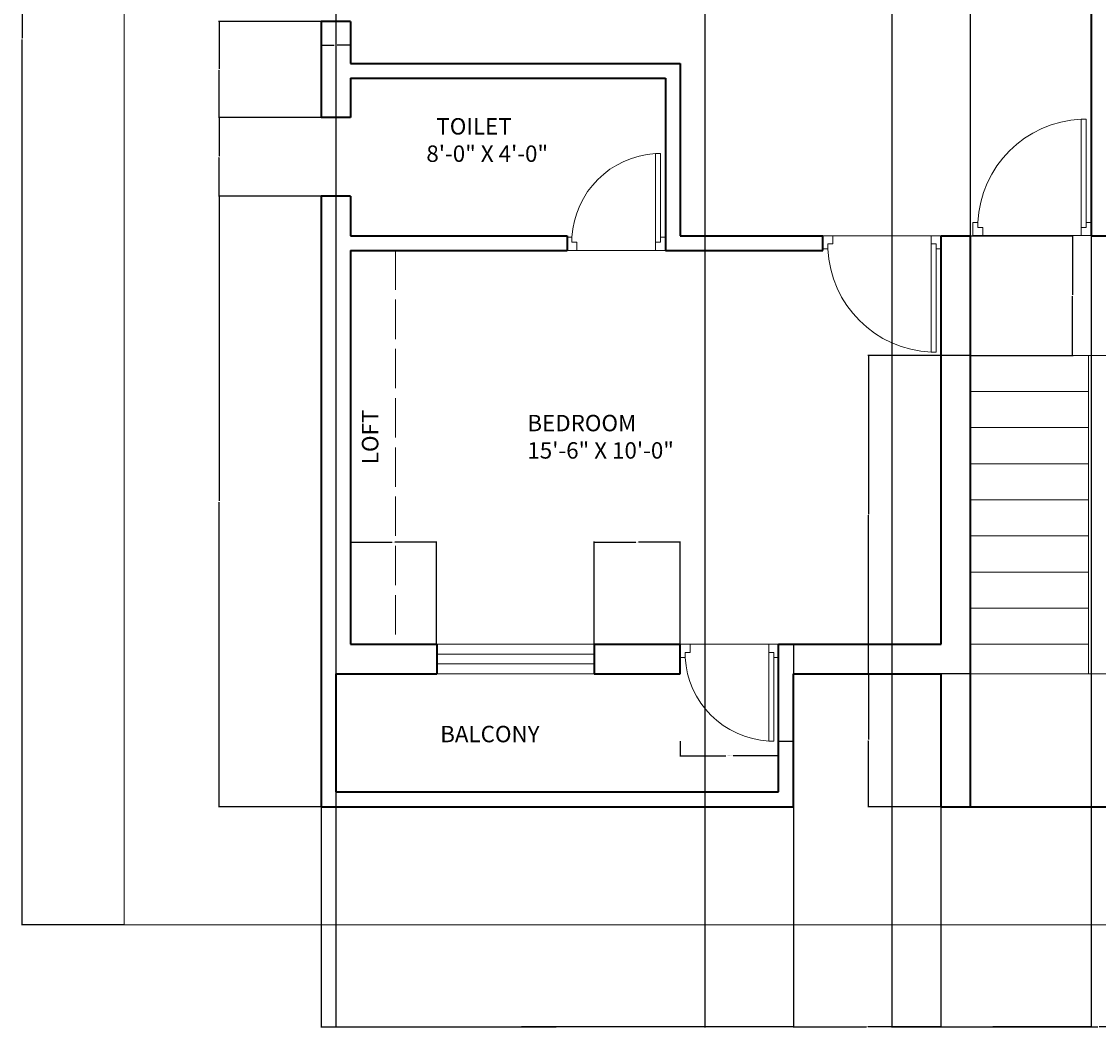
# Model space of a CAD drawing. Units: inches. Extents: x 3263 to 3926, y 954 to 1556.
# Tile 1 of 3: x 3263 to 3592, y 954 to 1260. Entities that reach past the tile are written whole.
import ezdxf

# ---------------------------------------------------------------- set-up
doc = ezdxf.new("R2010")
doc.units = ezdxf.units.IN
doc.linetypes.add('ACAD_ISO02W100', pattern=[15, 12, -3])
for name, color, linetype, lineweight in [('A-ANNO-DIMS', 2, 'Continuous', 18), ('A-ANNO-TEXT', 7, 'Continuous', 18), ('A-AREA-IDEN', 7, 'Continuous', 18), ('A-FLOR-OVHD', 8, 'ACAD_ISO02W100', 13), ('C-PROP', 8, 'Continuous', 18), ('door', 30, 'Continuous', 18), ('staircase', 31, 'Continuous', 18), ('wall', 7, 'Continuous', 35), ('window', 92, 'Continuous', 18)]:
    doc.layers.add(name, color=color, linetype=linetype, lineweight=lineweight)
doc.styles.get("Standard").update_dxf_attribs({"font": 'arial.ttf'})
doc.dimstyles.get("Standard").update_dxf_attribs({"dimtxt": 0.18, "dimasz": 0.18, "dimexe": 0.18, "dimexo": 0.0625, "dimgap": 0.09, "dimtad": 0, "dimtih": 1, "dimtoh": 1, "dimdec": 4, "dimzin": 0, "dimdsep": 46, "dimtxsty": 'Standard', "dimcen": 0.09, "dimadec": 0, "dimazin": 0, "dimtfac": 1, "dimtdec": 4, "dimtofl": 0, "dimtmove": 0, "dimatfit": 3, "dimfxl": 1, "dimtolj": 1, "dimtzin": 0, "dimarcsym": 0})

# ---------------------------------------------------------------- blocks, each defined once
blk = doc.blocks.new('d2')
at = {"layer": 'door'}
blk.add_line((4131.56, 1215.38), (4161.56, 1215.38), dxfattribs=at)
blk.add_lwpolyline([(4133.06, 1217.88), (4134.56, 1217.88), (4134.56, 1244.88), (4133.06, 1244.88)], close=True, dxfattribs=at)
for points in [[(4134.56, 1215.38), (4131.56, 1215.38), (4131.56, 1219.38), (4133.06, 1219.38), (4133.06, 1217.88), (4134.56, 1217.88), (4134.56, 1215.38)], [(4158.56, 1215.38), (4161.56, 1215.38), (4161.56, 1219.38), (4160.06, 1219.38), (4160.06, 1217.88), (4158.56, 1217.88), (4158.56, 1215.38)]]:
    blk.add_lwpolyline(points, dxfattribs=at)
blk.add_arc((4133.06, 1217.88), 27.04, 3.1798, 86.8202, dxfattribs=at)
blk = doc.blocks.new('w1')
at = {"layer": 'window'}
for p, q in [((3981.35, 1421.04), (3981.35, 1373.04)), ((3984.35, 1421.04), (3984.35, 1373.04))]:
    blk.add_line(p, q, dxfattribs=at)
blk.add_lwpolyline([(3978.35, 1373.04), (3987.35, 1373.04), (3987.35, 1421.04), (3978.35, 1421.04)], close=True, dxfattribs=at)
blk = doc.blocks.new('d1')
at = {"layer": 'door'}
blk.add_line((4131.56, 1272.79), (4167.56, 1272.79), dxfattribs=at)
blk.add_lwpolyline([(4133.06, 1275.29), (4134.56, 1275.29), (4134.56, 1308.29), (4133.06, 1308.29)], close=True, dxfattribs=at)
for points in [[(4134.56, 1272.79), (4131.56, 1272.79), (4131.56, 1276.79), (4133.06, 1276.79), (4133.06, 1275.29), (4134.56, 1275.29), (4134.56, 1272.79)], [(4164.56, 1272.79), (4167.56, 1272.79), (4167.56, 1276.79), (4166.06, 1276.79), (4166.06, 1275.29), (4164.56, 1275.29), (4164.56, 1272.79)]]:
    blk.add_lwpolyline(points, dxfattribs=at)
blk.add_arc((4133.06, 1275.29), 33.03, 2.6026, 87.3974, dxfattribs=at)
blk = doc.blocks.new('*D8')
at = {"layer": 'A-ANNO-DIMS', "color": 0, "lineweight": -2, "transparency": 16777216}
for p, q in [((3464.17, 1040.87), (3464.17, 1036.25)), ((3494.17, 1040.87), (3494.17, 1036.25)), ((3464.35, 1036.43), (3478.04, 1036.43)), ((3493.99, 1036.43), (3480.31, 1036.43))]:
    blk.add_line(p, q, dxfattribs=at)
at = {"layer": 'A-ANNO-DIMS', "color": 0, "transparency": 16777216}
for points in [[(3464.35, 1036.46), (3464.35, 1036.4), (3464.17, 1036.43)], [(3493.99, 1036.46), (3493.99, 1036.4), (3494.17, 1036.43)]]:
    blk.add_solid(points, dxfattribs=at)
at = {"layer": 'Defpoints', "color": 0, "transparency": 16777216}
for p in [(3464.17, 1040.93), (3494.17, 1040.93), (3464.17, 1036.43)]:
    blk.add_point(p, dxfattribs=at)
at = {"layer": 'A-ANNO-DIMS', "color": 0, "transparency": 16777216, "insert": (3479.17, 1036.43), "char_height": 0.18, "attachment_point": 5}
blk.add_mtext('\\A1;DOOR D2 30 TYP.', dxfattribs=at)
blk = doc.blocks.new('*D9')
at = {"layer": 'A-ANNO-DIMS', "color": 0, "lineweight": -2, "transparency": 16777216}
for p, q in [((3494.24, 1070.43), (3498.85, 1070.43)), ((3498.67, 1070.25), (3498.67, 1055.86)), ((3498.67, 1041.11), (3498.67, 1055.5)), ((3494.24, 1040.93), (3498.85, 1040.93))]:
    blk.add_line(p, q, dxfattribs=at)
at = {"layer": 'A-ANNO-DIMS', "color": 0, "transparency": 16777216}
for points in [[(3498.64, 1070.25), (3498.7, 1070.25), (3498.67, 1070.43)], [(3498.64, 1041.11), (3498.7, 1041.11), (3498.67, 1040.93)]]:
    blk.add_solid(points, dxfattribs=at)
at = {"layer": 'Defpoints', "color": 0, "transparency": 16777216}
for p in [(3494.17, 1070.43), (3494.17, 1040.93), (3498.67, 1040.93)]:
    blk.add_point(p, dxfattribs=at)
at = {"layer": 'A-ANNO-DIMS', "color": 0, "transparency": 16777216, "insert": (3498.67, 1055.68), "char_height": 0.18, "attachment_point": 5}
blk.add_mtext('\\A1;30 TYP.', dxfattribs=at)
blk = doc.blocks.new('*D11')
at = {"layer": 'A-ANNO-DIMS', "color": 0, "lineweight": -2, "transparency": 16777216}
for p, q in [((3354.67, 1260.12), (3354.67, 1252.8)), ((3363.67, 1260.12), (3363.67, 1252.8)), ((3354.85, 1252.98), (3358.72, 1252.98)), ((3363.49, 1252.98), (3359.63, 1252.98))]:
    blk.add_line(p, q, dxfattribs=at)
at = {"layer": 'A-ANNO-DIMS', "color": 0, "transparency": 16777216}
for points in [[(3354.85, 1253.01), (3354.85, 1252.95), (3354.67, 1252.98)], [(3363.49, 1253.01), (3363.49, 1252.95), (3363.67, 1252.98)]]:
    blk.add_solid(points, dxfattribs=at)
at = {"layer": 'Defpoints', "color": 0, "transparency": 16777216}
for p in [(3354.67, 1260.18), (3363.67, 1260.18), (3363.67, 1252.98)]:
    blk.add_point(p, dxfattribs=at)
at = {"layer": 'A-ANNO-DIMS', "color": 0, "transparency": 16777216, "insert": (3359.17, 1252.98), "char_height": 0.18, "attachment_point": 5}
blk.add_mtext('\\A1;9 TYP.', dxfattribs=at)
blk = doc.blocks.new('*D17')
at = {"layer": 'A-ANNO-DIMS', "color": 0, "lineweight": -2, "transparency": 16777216}
for p, q in [((3294.61, 1524.93), (3263.39, 1524.93)), ((3263.57, 1524.75), (3263.57, 1255.11)), ((3263.57, 985.11), (3263.57, 1254.75)), ((3294.61, 984.93), (3263.39, 984.93))]:
    blk.add_line(p, q, dxfattribs=at)
at = {"layer": 'A-ANNO-DIMS', "color": 0, "transparency": 16777216}
for points in [[(3263.54, 1524.75), (3263.6, 1524.75), (3263.57, 1524.93)], [(3263.54, 985.11), (3263.6, 985.11), (3263.57, 984.93)]]:
    blk.add_solid(points, dxfattribs=at)
at = {"layer": 'Defpoints', "color": 0, "transparency": 16777216}
for p in [(3263.57, 1524.93), (3294.67, 1524.93), (3294.67, 984.93)]:
    blk.add_point(p, dxfattribs=at)
at = {"layer": 'A-ANNO-DIMS', "color": 0, "transparency": 16777216, "insert": (3263.57, 1254.93), "char_height": 0.18, "attachment_point": 5}
blk.add_mtext('\\A1;540', dxfattribs=at)
blk = doc.blocks.new('*D24')
at = {"layer": 'A-ANNO-DIMS', "color": 0, "lineweight": -2, "transparency": 16777216}
for p, q in [((3354.67, 1020.87), (3354.67, 953.65)), ((3498.67, 1020.87), (3498.67, 953.65)), ((3354.85, 953.83), (3426.39, 953.83)), ((3498.49, 953.83), (3426.95, 953.83))]:
    blk.add_line(p, q, dxfattribs=at)
at = {"layer": 'A-ANNO-DIMS', "color": 0, "transparency": 16777216}
for points in [[(3354.85, 953.86), (3354.85, 953.8), (3354.67, 953.83)], [(3498.49, 953.86), (3498.49, 953.8), (3498.67, 953.83)]]:
    blk.add_solid(points, dxfattribs=at)
at = {"layer": 'Defpoints', "color": 0, "transparency": 16777216}
for p in [(3354.67, 1020.93), (3498.67, 1020.93), (3498.67, 953.83)]:
    blk.add_point(p, dxfattribs=at)
at = {"layer": 'A-ANNO-DIMS', "color": 0, "transparency": 16777216, "insert": (3426.67, 953.83), "char_height": 0.18, "attachment_point": 5}
blk.add_mtext('\\A1;144', dxfattribs=at)
blk = doc.blocks.new('*D25')
at = {"layer": 'A-ANNO-DIMS', "color": 0, "lineweight": -2, "transparency": 16777216}
for p, q in [((3498.67, 1020.87), (3498.67, 953.65)), ((3543.67, 1020.87), (3543.67, 953.65)), ((3498.85, 953.83), (3520.95, 953.83)), ((3543.49, 953.83), (3521.4, 953.83))]:
    blk.add_line(p, q, dxfattribs=at)
at = {"layer": 'A-ANNO-DIMS', "color": 0, "transparency": 16777216}
for points in [[(3498.85, 953.86), (3498.85, 953.8), (3498.67, 953.83)], [(3543.49, 953.86), (3543.49, 953.8), (3543.67, 953.83)]]:
    blk.add_solid(points, dxfattribs=at)
at = {"layer": 'Defpoints', "color": 0, "transparency": 16777216}
for p in [(3498.67, 1020.93), (3543.67, 1020.93), (3543.67, 953.83)]:
    blk.add_point(p, dxfattribs=at)
at = {"layer": 'A-ANNO-DIMS', "color": 0, "transparency": 16777216, "insert": (3521.17, 953.83), "char_height": 0.18, "attachment_point": 5}
blk.add_mtext('\\A1;45', dxfattribs=at)
blk = doc.blocks.new('*D26')
at = {"layer": 'A-ANNO-DIMS', "color": 0, "lineweight": -2, "transparency": 16777216}
for p, q in [((3543.67, 1020.87), (3543.67, 953.65)), ((3639.67, 1020.87), (3639.67, 953.65)), ((3543.85, 953.83), (3591.46, 953.83)), ((3639.49, 953.83), (3591.89, 953.83))]:
    blk.add_line(p, q, dxfattribs=at)
at = {"layer": 'A-ANNO-DIMS', "color": 0, "transparency": 16777216}
for points in [[(3543.85, 953.86), (3543.85, 953.8), (3543.67, 953.83)], [(3639.49, 953.86), (3639.49, 953.8), (3639.67, 953.83)]]:
    blk.add_solid(points, dxfattribs=at)
at = {"layer": 'Defpoints', "color": 0, "transparency": 16777216}
for p in [(3543.67, 1020.93), (3639.67, 1020.93), (3639.67, 953.83)]:
    blk.add_point(p, dxfattribs=at)
at = {"layer": 'A-ANNO-DIMS', "color": 0, "transparency": 16777216, "insert": (3591.67, 953.83), "char_height": 0.18, "attachment_point": 5}
blk.add_mtext('\\A1;96', dxfattribs=at)
blk = doc.blocks.new('*D29')
at = {"layer": 'A-ANNO-DIMS', "color": 0, "lineweight": -2, "transparency": 16777216}
for p, q in [((3552.67, 1020.99), (3552.67, 1556.21)), ((3630.67, 1020.99), (3630.67, 1556.21)), ((3552.85, 1556.03), (3591.46, 1556.03)), ((3630.49, 1556.03), (3591.89, 1556.03))]:
    blk.add_line(p, q, dxfattribs=at)
at = {"layer": 'A-ANNO-DIMS', "color": 0, "transparency": 16777216}
for points in [[(3552.85, 1556.06), (3552.85, 1556), (3552.67, 1556.03)], [(3630.49, 1556.06), (3630.49, 1556), (3630.67, 1556.03)]]:
    blk.add_solid(points, dxfattribs=at)
at = {"layer": 'Defpoints', "color": 0, "transparency": 16777216}
for p in [(3630.67, 1556.03), (3552.67, 1020.93), (3630.67, 1020.93)]:
    blk.add_point(p, dxfattribs=at)
at = {"layer": 'A-ANNO-DIMS', "color": 0, "transparency": 16777216, "insert": (3591.67, 1556.03), "char_height": 0.18, "attachment_point": 5}
blk.add_mtext('\\A1;78', dxfattribs=at)
blk = doc.blocks.new('*D30')
at = {"layer": 'A-ANNO-DIMS', "color": 0, "lineweight": -2, "transparency": 16777216}
for p, q in [((3552.61, 1158.43), (3521.39, 1158.43)), ((3521.57, 1158.25), (3521.57, 1110.11)), ((3521.57, 1061.61), (3521.57, 1109.75)), ((3552.61, 1061.43), (3521.39, 1061.43))]:
    blk.add_line(p, q, dxfattribs=at)
at = {"layer": 'A-ANNO-DIMS', "color": 0, "transparency": 16777216}
for points in [[(3521.54, 1158.25), (3521.6, 1158.25), (3521.57, 1158.43)], [(3521.54, 1061.61), (3521.6, 1061.61), (3521.57, 1061.43)]]:
    blk.add_solid(points, dxfattribs=at)
at = {"layer": 'Defpoints', "color": 0, "transparency": 16777216}
for p in [(3521.57, 1158.43), (3552.67, 1158.43), (3552.67, 1061.43)]:
    blk.add_point(p, dxfattribs=at)
at = {"layer": 'A-ANNO-DIMS', "color": 0, "transparency": 16777216, "insert": (3521.57, 1109.93), "char_height": 0.18, "attachment_point": 5}
blk.add_mtext('\\A1;97', dxfattribs=at)
blk = doc.blocks.new('*D31')
at = {"layer": 'A-ANNO-DIMS', "color": 0, "lineweight": -2, "transparency": 16777216}
for p, q in [((3552.74, 1194.93), (3583.95, 1194.93)), ((3583.77, 1194.75), (3583.77, 1176.86)), ((3583.77, 1158.61), (3583.77, 1176.5)), ((3552.74, 1158.43), (3583.95, 1158.43))]:
    blk.add_line(p, q, dxfattribs=at)
at = {"layer": 'A-ANNO-DIMS', "color": 0, "transparency": 16777216}
for points in [[(3583.74, 1194.75), (3583.8, 1194.75), (3583.77, 1194.93)], [(3583.74, 1158.61), (3583.8, 1158.61), (3583.77, 1158.43)]]:
    blk.add_solid(points, dxfattribs=at)
at = {"layer": 'Defpoints', "color": 0, "transparency": 16777216}
for p in [(3552.67, 1194.93), (3552.67, 1158.43), (3583.77, 1158.43)]:
    blk.add_point(p, dxfattribs=at)
at = {"layer": 'A-ANNO-DIMS', "color": 0, "transparency": 16777216, "insert": (3583.77, 1176.68), "char_height": 0.18, "attachment_point": 5}
blk.add_mtext('\\A1;36.5', dxfattribs=at)
blk = doc.blocks.new('*D32')
at = {"layer": 'A-ANNO-DIMS', "color": 0, "lineweight": -2, "transparency": 16777216}
for p, q in [((3552.61, 1061.43), (3521.39, 1061.43)), ((3521.57, 1061.25), (3521.57, 1041.36)), ((3521.57, 1021.11), (3521.57, 1041)), ((3552.61, 1020.93), (3521.39, 1020.93))]:
    blk.add_line(p, q, dxfattribs=at)
at = {"layer": 'A-ANNO-DIMS', "color": 0, "transparency": 16777216}
for points in [[(3521.54, 1061.25), (3521.6, 1061.25), (3521.57, 1061.43)], [(3521.54, 1021.11), (3521.6, 1021.11), (3521.57, 1020.93)]]:
    blk.add_solid(points, dxfattribs=at)
at = {"layer": 'Defpoints', "color": 0, "transparency": 16777216}
for p in [(3521.57, 1061.43), (3552.67, 1061.43), (3552.67, 1020.93)]:
    blk.add_point(p, dxfattribs=at)
at = {"layer": 'A-ANNO-DIMS', "color": 0, "transparency": 16777216, "insert": (3521.57, 1041.18), "char_height": 0.18, "attachment_point": 5}
blk.add_mtext('\\A1;40.5', dxfattribs=at)
blk = doc.blocks.new('*D36')
at = {"layer": 'A-ANNO-DIMS', "color": 0, "lineweight": -2, "transparency": 16777216}
for p, q in [((3359.17, 1484.37), (3359.17, 953.65)), ((3471.67, 1484.37), (3471.67, 953.65)), ((3359.35, 953.83), (3415.04, 953.83)), ((3471.49, 953.83), (3415.81, 953.83))]:
    blk.add_line(p, q, dxfattribs=at)
at = {"layer": 'A-ANNO-DIMS', "color": 0, "transparency": 16777216}
for points in [[(3359.35, 953.86), (3359.35, 953.8), (3359.17, 953.83)], [(3471.49, 953.86), (3471.49, 953.8), (3471.67, 953.83)]]:
    blk.add_solid(points, dxfattribs=at)
at = {"layer": 'Defpoints', "color": 0, "transparency": 16777216}
for p in [(3359.17, 1484.43), (3471.67, 1484.43), (3471.67, 953.83)]:
    blk.add_point(p, dxfattribs=at)
at = {"layer": 'A-ANNO-DIMS', "color": 0, "transparency": 16777216, "insert": (3415.42, 953.83), "char_height": 0.18, "attachment_point": 5}
blk.add_mtext('\\A1;112.5', dxfattribs=at)
blk = doc.blocks.new('*D38')
at = {"layer": 'A-ANNO-DIMS', "color": 0, "lineweight": -2, "transparency": 16777216}
for p, q in [((3528.67, 1484.37), (3528.67, 953.65)), ((3589.42, 1484.37), (3589.42, 953.65)), ((3528.85, 953.83), (3558.65, 953.83)), ((3589.24, 953.83), (3559.44, 953.83))]:
    blk.add_line(p, q, dxfattribs=at)
at = {"layer": 'A-ANNO-DIMS', "color": 0, "transparency": 16777216}
for points in [[(3528.85, 953.86), (3528.85, 953.8), (3528.67, 953.83)], [(3589.24, 953.86), (3589.24, 953.8), (3589.42, 953.83)]]:
    blk.add_solid(points, dxfattribs=at)
at = {"layer": 'Defpoints', "color": 0, "transparency": 16777216}
for p in [(3528.67, 1484.43), (3589.42, 1484.43), (3589.42, 953.83)]:
    blk.add_point(p, dxfattribs=at)
at = {"layer": 'A-ANNO-DIMS', "color": 0, "transparency": 16777216, "insert": (3559.05, 953.83), "char_height": 0.18, "attachment_point": 5}
blk.add_mtext('\\A1;60.75', dxfattribs=at)
blk = doc.blocks.new('*D49')
at = {"layer": 'A-ANNO-DIMS', "color": 0, "lineweight": -2, "transparency": 16777216}
for p, q in [((3354.61, 1260.18), (3323.39, 1260.18)), ((3323.57, 1260), (3323.57, 1245.74)), ((3323.57, 1231.11), (3323.57, 1245.37)), ((3354.61, 1230.93), (3323.39, 1230.93))]:
    blk.add_line(p, q, dxfattribs=at)
at = {"layer": 'A-ANNO-DIMS', "color": 0, "transparency": 16777216}
for points in [[(3323.54, 1260), (3323.6, 1260), (3323.57, 1260.18)], [(3323.54, 1231.11), (3323.6, 1231.11), (3323.57, 1230.93)]]:
    blk.add_solid(points, dxfattribs=at)
at = {"layer": 'Defpoints', "color": 0, "transparency": 16777216}
for p in [(3323.57, 1260.18), (3354.67, 1260.18), (3354.67, 1230.93)]:
    blk.add_point(p, dxfattribs=at)
at = {"layer": 'A-ANNO-DIMS', "color": 0, "transparency": 16777216, "insert": (3323.57, 1245.56), "char_height": 0.18, "attachment_point": 5}
blk.add_mtext('\\A1;29.25', dxfattribs=at)
blk = doc.blocks.new('*D50')
at = {"layer": 'A-ANNO-DIMS', "color": 0, "lineweight": -2, "transparency": 16777216}
for p, q in [((3354.61, 1230.93), (3323.39, 1230.93)), ((3323.57, 1230.75), (3323.57, 1219.11)), ((3323.57, 1207.11), (3323.57, 1218.75)), ((3354.61, 1206.93), (3323.39, 1206.93))]:
    blk.add_line(p, q, dxfattribs=at)
at = {"layer": 'A-ANNO-DIMS', "color": 0, "transparency": 16777216}
for points in [[(3323.54, 1230.75), (3323.6, 1230.75), (3323.57, 1230.93)], [(3323.54, 1207.11), (3323.6, 1207.11), (3323.57, 1206.93)]]:
    blk.add_solid(points, dxfattribs=at)
at = {"layer": 'Defpoints', "color": 0, "transparency": 16777216}
for p in [(3323.57, 1230.93), (3354.67, 1230.93), (3354.67, 1206.93)]:
    blk.add_point(p, dxfattribs=at)
at = {"layer": 'A-ANNO-DIMS', "color": 0, "transparency": 16777216, "insert": (3323.57, 1218.93), "char_height": 0.18, "attachment_point": 5}
blk.add_mtext('\\A1;24', dxfattribs=at)
blk = doc.blocks.new('*D51')
at = {"layer": 'A-ANNO-DIMS', "color": 0, "lineweight": -2, "transparency": 16777216}
for p, q in [((3354.61, 1206.93), (3323.39, 1206.93)), ((3323.57, 1206.75), (3323.57, 1114.11)), ((3323.57, 1021.11), (3323.57, 1113.75)), ((3354.61, 1020.93), (3323.39, 1020.93))]:
    blk.add_line(p, q, dxfattribs=at)
at = {"layer": 'A-ANNO-DIMS', "color": 0, "transparency": 16777216}
for points in [[(3323.54, 1206.75), (3323.6, 1206.75), (3323.57, 1206.93)], [(3323.54, 1021.11), (3323.6, 1021.11), (3323.57, 1020.93)]]:
    blk.add_solid(points, dxfattribs=at)
at = {"layer": 'Defpoints', "color": 0, "transparency": 16777216}
for p in [(3323.57, 1206.93), (3354.67, 1206.93), (3354.67, 1020.93)]:
    blk.add_point(p, dxfattribs=at)
at = {"layer": 'A-ANNO-DIMS', "color": 0, "transparency": 16777216, "insert": (3323.57, 1113.93), "char_height": 0.18, "attachment_point": 5}
blk.add_mtext('\\A1;186', dxfattribs=at)
blk = doc.blocks.new('*D52')
at = {"layer": 'A-ANNO-DIMS', "color": 0, "lineweight": -2, "transparency": 16777216}
for p, q in [((3363.67, 1070.49), (3363.67, 1101.71)), ((3363.85, 1101.53), (3376.4, 1101.53)), ((3389.74, 1101.53), (3377.2, 1101.53)), ((3389.92, 1070.49), (3389.92, 1101.71))]:
    blk.add_line(p, q, dxfattribs=at)
at = {"layer": 'A-ANNO-DIMS', "color": 0, "transparency": 16777216}
for points in [[(3363.85, 1101.56), (3363.85, 1101.5), (3363.67, 1101.53)], [(3389.74, 1101.56), (3389.74, 1101.5), (3389.92, 1101.53)]]:
    blk.add_solid(points, dxfattribs=at)
at = {"layer": 'Defpoints', "color": 0, "transparency": 16777216}
for p in [(3389.92, 1101.53), (3363.67, 1070.43), (3389.92, 1070.43)]:
    blk.add_point(p, dxfattribs=at)
at = {"layer": 'A-ANNO-DIMS', "color": 0, "transparency": 16777216, "insert": (3376.8, 1101.53), "char_height": 0.18, "attachment_point": 5}
blk.add_mtext('\\A1;26.25', dxfattribs=at)
blk = doc.blocks.new('*D53')
at = {"layer": 'A-ANNO-DIMS', "color": 0, "lineweight": -2, "transparency": 16777216}
for p, q in [((3437.92, 1070.49), (3437.92, 1101.71)), ((3438.1, 1101.53), (3450.65, 1101.53)), ((3463.99, 1101.53), (3451.45, 1101.53)), ((3464.17, 1070.49), (3464.17, 1101.71))]:
    blk.add_line(p, q, dxfattribs=at)
at = {"layer": 'A-ANNO-DIMS', "color": 0, "transparency": 16777216}
for points in [[(3438.1, 1101.56), (3438.1, 1101.5), (3437.92, 1101.53)], [(3463.99, 1101.56), (3463.99, 1101.5), (3464.17, 1101.53)]]:
    blk.add_solid(points, dxfattribs=at)
at = {"layer": 'Defpoints', "color": 0, "transparency": 16777216}
for p in [(3464.17, 1101.53), (3437.92, 1070.43), (3464.17, 1070.43)]:
    blk.add_point(p, dxfattribs=at)
at = {"layer": 'A-ANNO-DIMS', "color": 0, "transparency": 16777216, "insert": (3451.05, 1101.53), "char_height": 0.18, "attachment_point": 5}
blk.add_mtext('\\A1;26.25', dxfattribs=at)

msp = doc.modelspace()

# ---------------------------------------------------------------- linework, layer by layer
at = {"layer": 'A-FLOR-OVHD'}
msp.add_line((3377.4044, 1190.4303), (3377.4044, 1070.4303), dxfattribs=at)
at = {"layer": 'C-PROP'}
for p, q in [((3294.6743, 1524.9303), (3294.6743, 984.9303)), ((3294.6743, 984.9303), (3894.6743, 984.9303))]:
    msp.add_line(p, q, dxfattribs=at)
at = {"layer": 'staircase'}
for p, q in [((3552.6743, 1158.4303), (3630.6743, 1158.4303)), ((3588.6743, 1061.4303), (3588.6743, 1158.4303)), ((3552.6743, 1147.4303), (3588.6743, 1147.4303)), ((3552.6743, 1136.4303), (3588.6743, 1136.4303)), ((3552.6743, 1125.4303), (3588.6743, 1125.4303)), ((3552.6743, 1114.4303), (3588.6743, 1114.4303)), ((3552.6743, 1103.4303), (3588.6743, 1103.4303)), ((3552.6743, 1092.4303), (3588.6743, 1092.4303)), ((3552.6743, 1081.4303), (3588.6743, 1081.4303)), ((3552.6743, 1070.4303), (3588.6743, 1070.4303)), ((3552.6743, 1061.4303), (3630.6743, 1061.4303))]:
    msp.add_line(p, q, dxfattribs=at)
at = {"layer": 'wall'}
for p, q in [((3589.4243, 1362.9303), (3589.4243, 1194.9303)), ((3363.6743, 1260.1803), (3354.6743, 1260.1803)), ((3354.6743, 1260.1803), (3354.6743, 1230.9303)), ((3363.6743, 1260.1803), (3363.6743, 1247.4303)), ((3363.6743, 1247.4303), (3464.1743, 1247.4303)), ((3464.1743, 1247.4303), (3464.1743, 1194.9303)), ((3363.6743, 1242.9303), (3459.6743, 1242.9303)), ((3363.6743, 1242.9303), (3363.6743, 1230.9303)), ((3459.6743, 1242.9303), (3459.6743, 1190.4303)), ((3363.6743, 1230.9303), (3354.6743, 1230.9303)), ((3363.6743, 1206.9303), (3354.6743, 1206.9303)), ((3354.6743, 1206.9303), (3354.6743, 1020.9303)), ((3363.6743, 1206.9303), (3363.6743, 1194.9303)), ((3363.6743, 1194.9303), (3429.6743, 1194.9303)), ((3429.6743, 1194.9303), (3429.6743, 1190.4303)), ((3464.1743, 1194.9303), (3507.6743, 1194.9303)), ((3507.6743, 1190.4303), (3507.6743, 1194.9303)), ((3543.6743, 1194.9303), (3552.6743, 1194.9303)), ((3543.6743, 1070.4303), (3543.6743, 1194.9303)), ((3552.6743, 1020.9303), (3552.6743, 1194.9303)), ((3589.4243, 1194.9303), (3593.9243, 1194.9303)), ((3363.6743, 1190.4303), (3429.6743, 1190.4303)), ((3363.6743, 1190.4303), (3363.6743, 1070.4303)), ((3459.6743, 1190.4303), (3464.1743, 1190.4303)), ((3464.1743, 1190.4303), (3507.6743, 1190.4303)), ((3363.6743, 1070.4303), (3389.9243, 1070.4303)), ((3389.9243, 1070.4303), (3389.9243, 1061.4303)), ((3437.9243, 1070.4303), (3437.9243, 1061.4303)), ((3437.9243, 1070.4303), (3464.1743, 1070.4303)), ((3464.1743, 1061.4303), (3464.1743, 1070.4303)), ((3494.1743, 1025.4303), (3494.1743, 1070.4303)), ((3494.1743, 1070.4303), (3543.6743, 1070.4303)), ((3359.1743, 1061.4303), (3389.9243, 1061.4303)), ((3359.1743, 1061.4303), (3359.1743, 1025.4303)), ((3437.9243, 1061.4303), (3464.1743, 1061.4303)), ((3498.6743, 1020.9303), (3498.6743, 1061.4303)), ((3498.6743, 1061.4303), (3543.6743, 1061.4303)), ((3543.6743, 1020.9303), (3543.6743, 1061.4303)), ((3359.1743, 1025.4303), (3494.1743, 1025.4303)), ((3354.6743, 1020.9303), (3498.6743, 1020.9303)), ((3543.6743, 1020.9303), (3639.6743, 1020.9303))]:
    msp.add_line(p, q, dxfattribs=at)

# ---------------------------------------------------------------- block references
at = {"layer": 'door', "xscale": -1}
for name, p in [('d1', (7720.9828, -77.8568)), ('d2', (7591.2328, -24.9474))]:
    msp.add_blockref(name, p, dxfattribs=at)
at = {"layer": 'door', "rotation": 180}
for name, p in [('d1', (7675.2328, 2467.7175)), ('d2', (7625.7328, 2285.808))]:
    msp.add_blockref(name, p, dxfattribs=at)
at = {"layer": 'window', "rotation": 270}
msp.add_blockref('w1', (2016.8872, 5048.7852), dxfattribs=at)

# ---------------------------------------------------------------- texts
at = {"layer": 'A-ANNO-TEXT', "insert": (3367.141, 1125.2869), "char_height": 5, "attachment_point": 1, "rotation": 90}
msp.add_mtext_dynamic_manual_height_columns('LOFT', width=62.092631, gutter_width=12.5, heights=[0], dxfattribs=at)
at = {"layer": 'A-AREA-IDEN', "char_height": 5, "attachment_point": 1}
for s, width, insert in [('  TOILET\\P8\'-0" X 4\'-0"', 42.17852, (3386.7807, 1230.7511)), ('BEDROOM\\P15\'-6" X 10\'-0"', 65.299351, (3417.5734, 1140.3257)), ('BALCONY', 62.092631, (3390.9994, 1045.5573))]:
    msp.add_mtext_dynamic_manual_height_columns(s, width=width, gutter_width=12.5, heights=[0], dxfattribs=dict(at, insert=insert))

# ---------------------------------------------------------------- dimensions: what is measured, and where the dimension line sits
at = {"layer": 'A-ANNO-DIMS'}
for base, p1, p2, override, picture, middle in [((3630.6743, 1556.0303), (3552.6743, 1020.9303), (3630.6743, 1020.9303), {"dimdec": 0, "dimlfac": 1, "dimrnd": 0, "dimzin": 0, "dimdsep": 46, "dimlunit": 2}, '*D29', (3591.6743, 1556.0303)), ((3471.6743, 953.8303), (3359.1743, 1484.4303), (3471.6743, 1484.4303), {"dimdec": 1, "dimlfac": 1, "dimrnd": 0, "dimzin": 0, "dimdsep": 46, "dimlunit": 2}, '*D36', (3415.4243, 953.8303)), ((3589.4243, 953.8303), (3528.6743, 1484.4303), (3589.4243, 1484.4303), {"dimdec": 2, "dimlfac": 1, "dimrnd": 0, "dimzin": 0, "dimdsep": 46, "dimlunit": 2}, '*D38', (3559.0493, 953.8303)), ((3389.9243, 1101.5303), (3363.6743, 1070.4303), (3389.9243, 1070.4303), {"dimdec": 2, "dimlfac": 1, "dimrnd": 0, "dimzin": 0, "dimdsep": 46, "dimlunit": 2}, '*D52', (3376.7993, 1101.5303)), ((3498.6743, 953.8303), (3354.6743, 1020.9303), (3498.6743, 1020.9303), {"dimdec": 0, "dimlfac": 1, "dimrnd": 0, "dimzin": 0, "dimdsep": 46, "dimlunit": 2}, '*D24', (3426.6743, 953.8303)), ((3543.6743, 953.8303), (3498.6743, 1020.9303), (3543.6743, 1020.9303), {"dimdec": 0, "dimlfac": 1, "dimrnd": 0, "dimzin": 0, "dimdsep": 46, "dimlunit": 2}, '*D25', (3521.1743, 953.8303)), ((3639.6743, 953.8303), (3543.6743, 1020.9303), (3639.6743, 1020.9303), {"dimdec": 0, "dimlfac": 1, "dimrnd": 0, "dimzin": 0, "dimdsep": 46, "dimlunit": 2}, '*D26', (3591.6743, 953.8303))]:
    dim = msp.add_linear_dim(base=base, p1=p1, p2=p2, dimstyle='Standard', override=override, dxfattribs=at)
    dim.commit()
    dim.dimension.update_dxf_attribs({"geometry": picture, "text_midpoint": middle})
for base, p1, p2, angle, override, picture, middle in [((3263.5743, 1524.9303), (3294.6743, 984.9303), (3294.6743, 1524.9303), 90, {"dimdec": 0, "dimlfac": 1, "dimrnd": 0, "dimzin": 0, "dimdsep": 46, "dimlunit": 2}, '*D17', (3263.5743, 1254.9303)), ((3323.5743, 1260.1803), (3354.6743, 1230.9303), (3354.6743, 1260.1803), 90, {"dimdec": 2, "dimlfac": 1, "dimrnd": 0, "dimzin": 0, "dimdsep": 46, "dimlunit": 2}, '*D49', (3323.5743, 1245.5553)), ((3323.5743, 1230.9303), (3354.6743, 1206.9303), (3354.6743, 1230.9303), 90, {"dimdec": 0, "dimlfac": 1, "dimrnd": 0, "dimzin": 0, "dimdsep": 46, "dimlunit": 2}, '*D50', (3323.5743, 1218.9303)), ((3323.5743, 1206.9303), (3354.6743, 1020.9303), (3354.6743, 1206.9303), 90, {"dimdec": 0, "dimlfac": 1, "dimrnd": 0, "dimzin": 0, "dimdsep": 46, "dimlunit": 2}, '*D51', (3323.5743, 1113.9303)), ((3583.7743, 1158.4303), (3552.6743, 1194.9303), (3552.6743, 1158.4303), 270, {"dimdec": 1, "dimlfac": 1, "dimrnd": 0, "dimzin": 0, "dimdsep": 46, "dimlunit": 2}, '*D31', (3583.7743, 1176.6803)), ((3521.5743, 1158.4303), (3552.6743, 1061.4303), (3552.6743, 1158.4303), 90, {"dimdec": 0, "dimlfac": 1, "dimrnd": 0, "dimzin": 0, "dimdsep": 46, "dimlunit": 2}, '*D30', (3521.5743, 1109.9303)), ((3464.1743, 1101.5303), (3437.9243, 1070.4303), (3464.1743, 1070.4303), 0, {"dimdec": 2, "dimlfac": 1, "dimrnd": 0, "dimzin": 0, "dimdsep": 46, "dimlunit": 2}, '*D53', (3451.0493, 1101.5303)), ((3521.5743, 1061.4303), (3552.6743, 1020.9303), (3552.6743, 1061.4303), 90, {"dimdec": 1, "dimlfac": 1, "dimrnd": 0, "dimzin": 0, "dimdsep": 46, "dimlunit": 2}, '*D32', (3521.5743, 1041.1803))]:
    dim = msp.add_linear_dim(base=base, p1=p1, p2=p2, angle=angle, dimstyle='Standard', override=override, dxfattribs=at)
    dim.commit()
    dim.dimension.update_dxf_attribs({"geometry": picture, "text_midpoint": middle})
dim = msp.add_linear_dim(base=(3363.6743, 1252.9803), p1=(3354.6743, 1260.1803), p2=(3363.6743, 1260.1803), text='<> TYP.', dimstyle='Standard', override={"dimdec": 0, "dimlfac": 1, "dimrnd": 0, "dimzin": 0, "dimdsep": 46, "dimlunit": 2}, dxfattribs=at)
dim.commit()
dim.dimension.update_dxf_attribs({"geometry": '*D11', "text_midpoint": (3359.1743, 1252.9803)})
for base, p1, p2, angle, text, picture, middle in [((3498.6742660714, 1040.9303250292), (3494.1742660714, 1070.4303250292), (3494.1742660714, 1040.9303250292), 270, '<> TYP.', '*D9', (3498.6742660714, 1055.6803250292)), ((3464.1743, 1036.4303), (3494.1743, 1040.9303), (3464.1743, 1040.9303), 180, 'DOOR D2 <> TYP.', '*D8', (3479.1743, 1036.4303))]:
    dim = msp.add_linear_dim(base=base, p1=p1, p2=p2, angle=angle, text=text, dimstyle='Standard', override={"dimdec": 0, "dimlfac": 1, "dimrnd": 0, "dimzin": 0, "dimdsep": 46, "dimlunit": 2}, dxfattribs=at)
    dim.commit()
    dim.dimension.update_dxf_attribs({"geometry": picture, "text_midpoint": middle})

doc.saveas('drawing.dxf')
